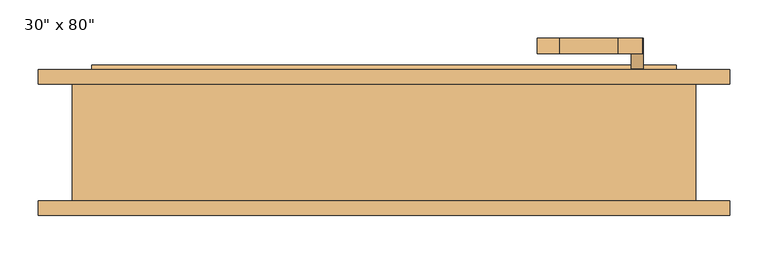
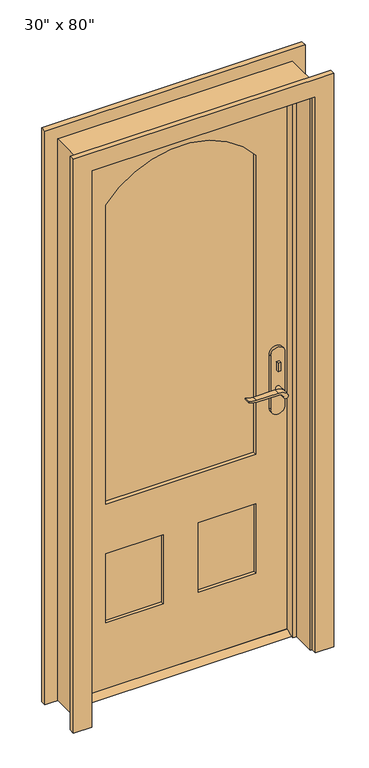
"""IFC4 building model written with IfcOpenShell, lengths in millimetres: door geometry."""

from ifc_helpers import new_model, si_unit, point, frame, frame_2d, origin, place, context, project, spatial, polyline, circle_curve, trimmed, segment, composite_curve, outline, extrude, faceted_brep, source, transform, mapped, element, save


def door_14b9be53(model_context):
    return source(origin(), model_context, "Body", "SolidModel", [
        extrude(outline(polyline([(38.1, 12.7), (73.025, 12.7), (98.425, 0.0), (12.7, 0.0), (38.1, 12.7)])), frame((-381.0, 0.0, 0.0), z_axis=(1.0, 0.0, 0.0), x_axis=(0.0, 1.0, 0.0)), (0.0, 0.0, 1.0), 762.0),
        extrude(outline(polyline([(335.2, 18.1), (325.2, 18.1), (325.2, 28.1), (335.2, 28.1), (335.2, 18.1)])), frame((0.0, 0.0, 981.9), z_axis=(0.0, 0.0, 1.0), x_axis=(1.0, 0.0, 0.0)), (0.0, 0.0, 1.0), 30.0),
        extrude(outline(composite_curve([segment(trimmed(circle_curve(frame_2d((996.9, 330.2)), 8.0), [point((996.9, 322.2))], [point((996.9, 338.2))], False, "CARTESIAN"), True, "CONTINUOUS"), segment(trimmed(circle_curve(frame_2d((996.9, 330.2)), 8.0), [point((996.9, 338.2))], [point((996.9, 322.2))], False, "CARTESIAN"), True, "CONTINUOUS")], self_intersect=False)), frame((0.0, 83.025, 0.0), z_axis=(0.0, 1.0, 0.0), x_axis=(0.0, 0.0, 1.0)), (0.0, 0.0, 1.0), 10.0),
        extrude(outline(composite_curve([segment(trimmed(circle_curve(frame_2d((897.1555521, 306.5324871)), 37.2832219), [point((919.0523287, 336.7081363))], [point((934.4, 304.8325667))], False, "CARTESIAN"), True, "CONTINUOUS"), segment(polyline([(934.4, 304.8325667), (934.4, 228.5564091)]), True, "CONTINUOUS"), segment(trimmed(circle_curve(frame_2d((1017.6850638, 228.6227909)), 83.2850902), [point((934.4, 228.5564091))], [point((939.4, 200.2))], True, "CARTESIAN"), True, "CONTINUOUS"), segment(polyline([(939.4, 200.2), (936.6135558, 200.2)]), True, "CONTINUOUS"), segment(trimmed(circle_curve(frame_2d((986.6709207, 232.1396612)), 59.3791355), [point((936.6135558, 200.2))], [point((927.4, 228.5564091))], False, "CARTESIAN"), True, "CONTINUOUS"), segment(polyline([(927.4, 228.5564091), (927.4, 304.8138099)]), True, "CONTINUOUS"), segment(trimmed(circle_curve(frame_2d((909.2738613, 304.8138099)), 18.1261387), [point((927.4, 304.8138099))], [point((914.4, 322.2))], True, "CARTESIAN"), True, "CONTINUOUS"), segment(trimmed(circle_curve(frame_2d((914.4, 330.2)), 8.0), [point((914.4, 322.2))], [point((919.0523287, 336.7081363))], False, "CARTESIAN"), True, "CONTINUOUS")], self_intersect=False)), frame((0.0, -21.9, 0.0), z_axis=(0.0, 1.0, 0.0), x_axis=(0.0, 0.0, 1.0)), (0.0, 0.0, 1.0), 20.0),
        extrude(outline(composite_curve([segment(trimmed(circle_curve(frame_2d((914.4, 330.2)), 8.0), [point((914.3999903, 322.2))], [point((919.0523287, 336.7081363))], False, "CARTESIAN"), True, "CONTINUOUS"), segment(trimmed(circle_curve(frame_2d((897.1555521, 306.5324871)), 37.2832219), [point((919.0523287, 336.7081363))], [point((934.4, 304.8325667))], False, "CARTESIAN"), True, "CONTINUOUS"), segment(polyline([(934.4, 304.8325667), (934.4, 228.5564091)]), True, "CONTINUOUS"), segment(trimmed(circle_curve(frame_2d((1017.6850638, 228.6227909)), 83.2850902), [point((934.4, 228.5564091))], [point((939.4, 200.2))], True, "CARTESIAN"), True, "CONTINUOUS"), segment(polyline([(939.4, 200.2), (936.6135558, 200.2)]), True, "CONTINUOUS"), segment(trimmed(circle_curve(frame_2d((986.6709207, 232.1396612)), 59.3791355), [point((936.6135558, 200.2))], [point((927.4, 228.5564091))], False, "CARTESIAN"), True, "CONTINUOUS"), segment(polyline([(927.4, 228.5564091), (927.4, 304.8138122)]), True, "CONTINUOUS"), segment(trimmed(circle_curve(frame_2d((909.2738682, 304.8138122)), 18.1261318), [point((927.4, 304.8138122))], [point((914.3999903, 322.2))], True, "CARTESIAN"), True, "CONTINUOUS")], self_intersect=False)), frame((0.0, 113.025, 0.0), z_axis=(0.0, 1.0, 0.0), x_axis=(0.0, 0.0, 1.0)), (0.0, 0.0, 1.0), 20.0),
        extrude(outline(composite_curve([segment(trimmed(circle_curve(frame_2d((914.4, 330.2)), 8.0), [point((914.4, 322.2))], [point((914.4, 338.2))], False, "CARTESIAN"), True, "CONTINUOUS"), segment(trimmed(circle_curve(frame_2d((914.4, 330.2)), 8.0), [point((914.4, 338.2))], [point((914.4, 322.2))], False, "CARTESIAN"), True, "CONTINUOUS")], self_intersect=False)), frame((0.0, -1.9, 0.0), z_axis=(0.0, 1.0, 0.0), x_axis=(0.0, 0.0, 1.0)), (0.0, 0.0, 1.0), 30.0),
        extrude(outline(composite_curve([segment(trimmed(circle_curve(frame_2d((914.4, 330.2)), 8.0), [point((914.4, 322.2))], [point((914.4, 338.2))], False, "CARTESIAN"), True, "CONTINUOUS"), segment(trimmed(circle_curve(frame_2d((914.4, 330.2)), 8.0), [point((914.4, 338.2))], [point((914.4, 322.2))], False, "CARTESIAN"), True, "CONTINUOUS")], self_intersect=False)), frame((0.0, 83.025, 0.0), z_axis=(0.0, 1.0, 0.0), x_axis=(0.0, 0.0, 1.0)), (0.0, 0.0, 1.0), 30.0),
        extrude(outline(composite_curve([segment(polyline([(844.4, 355.2), (1039.4, 355.2)]), True, "CONTINUOUS"), segment(trimmed(circle_curve(frame_2d((1039.4, 330.2)), 25.0), [point((1039.4, 355.2))], [point((1039.4, 305.2))], False, "CARTESIAN"), True, "CONTINUOUS"), segment(polyline([(1039.4, 305.2), (844.4, 305.2)]), True, "CONTINUOUS"), segment(trimmed(circle_curve(frame_2d((844.4, 330.2)), 25.0), [point((844.4, 305.2))], [point((844.4, 355.2))], False, "CARTESIAN"), True, "CONTINUOUS")], self_intersect=False)), frame((0.0, 28.1, 0.0), z_axis=(0.0, 1.0, 0.0), x_axis=(0.0, 0.0, 1.0)), (0.0, 0.0, 1.0), 10.0),
        extrude(outline(composite_curve([segment(polyline([(844.4, 355.2), (1039.4, 355.2)]), True, "CONTINUOUS"), segment(trimmed(circle_curve(frame_2d((1039.4, 330.2)), 25.0), [point((1039.4, 355.2))], [point((1039.4, 305.2))], False, "CARTESIAN"), True, "CONTINUOUS"), segment(polyline([(1039.4, 305.2), (844.4, 305.2)]), True, "CONTINUOUS"), segment(trimmed(circle_curve(frame_2d((844.4, 330.2)), 25.0), [point((844.4, 305.2))], [point((844.4, 355.2))], False, "CARTESIAN"), True, "CONTINUOUS")], self_intersect=False)), frame((0.0, 73.025, 0.0), z_axis=(0.0, 1.0, 0.0), x_axis=(0.0, 0.0, 1.0)), (0.0, 0.0, 1.0), 10.0),
        extrude(outline(polyline([(2032.0, -381.0), (12.7, -381.0), (12.7, 381.0), (2032.0, 381.0), (2032.0, -381.0)]), holes=[composite_curve([segment(polyline([(688.975, -260.35), (1784.35, -260.35)]), True, "CONTINUOUS"), segment(trimmed(circle_curve(frame_2d((1580.99125, 0.0)), 330.35875), [point((1784.35, -260.35))], [point((1784.35, 260.35))], True, "CARTESIAN"), True, "CONTINUOUS"), segment(polyline([(1784.35, 260.35), (688.975, 260.35), (688.975, -260.35)]), True, "CONTINUOUS")], self_intersect=False), polyline([(508.0, -60.325), (254.0, -60.325), (254.0, -260.35), (508.0, -260.35), (508.0, -60.325)]), polyline([(508.0, 260.35), (254.0, 260.35), (254.0, 60.325), (508.0, 60.325), (508.0, 260.35)])]), frame((0.0, 38.1, 0.0), z_axis=(0.0, 1.0, 0.0), x_axis=(0.0, 0.0, 1.0)), (0.0, 0.0, 1.0), 34.925),
        faceted_brep([(406.4, 73.025, 0.0), (406.4, -79.375, 0.0), (381.0, -79.375, 0.0), (381.0, 3.175, 0.0), (368.3, 3.175, 0.0), (368.3, 38.1, 0.0), (381.0, 38.1, 0.0), (381.0, 73.025, 0.0), (406.4, 73.025, 2057.4), (406.4, -79.375, 2057.4), (-406.4, -79.375, 2057.4), (-406.4, -79.375, 0.0), (-381.0, -79.375, 0.0), (-381.0, -79.375, 2032.0), (381.0, -79.375, 2032.0), (381.0, 3.175, 2032.0), (-381.0, 3.175, 2032.0), (-381.0, 3.175, 0.0), (-368.3, 3.175, 0.0), (-368.3, 3.175, 2019.3), (368.3, 3.175, 2019.3), (368.3, 38.1, 2019.3), (-368.3, 38.1, 2019.3), (-368.3, 38.1, 0.0), (-381.0, 38.1, 0.0), (-381.0, 38.1, 2032.0), (381.0, 38.1, 2032.0), (381.0, 73.025, 2032.0), (-381.0, 73.025, 2032.0), (-381.0, 73.025, 0.0), (-406.4, 73.025, 0.0), (-406.4, 73.025, 2057.4)], [[[0, 1, 2, 3, 4, 5, 6, 7]], [[1, 0, 8, 9]], [[2, 1, 9, 10, 11, 12, 13, 14]], [[3, 2, 14, 15]], [[4, 3, 15, 16, 17, 18, 19, 20]], [[5, 4, 20, 21]], [[6, 5, 21, 22, 23, 24, 25, 26]], [[7, 6, 26, 27]], [[0, 7, 27, 28, 29, 30, 31, 8]], [[9, 8, 31, 10]], [[15, 14, 13, 16]], [[21, 20, 19, 22]], [[27, 26, 25, 28]], [[30, 29, 24, 23, 18, 17, 12, 11]], [[10, 31, 30, 11]], [[16, 13, 12, 17]], [[22, 19, 18, 23]], [[28, 25, 24, 29]]]),
        extrude(outline(polyline([(-60.325, 49.7416667), (-260.35, 49.7416667), (-260.35, 61.3833333), (-60.325, 61.3833333), (-60.325, 49.7416667)])), frame((0.0, 0.0, 254.0), z_axis=(0.0, 0.0, 1.0), x_axis=(1.0, 0.0, 0.0)), (0.0, 0.0, 1.0), 254.0),
        extrude(outline(polyline([(260.35, 49.7416667), (60.325, 49.7416667), (60.325, 61.3833333), (260.35, 61.3833333), (260.35, 49.7416667)])), frame((0.0, 0.0, 254.0), z_axis=(0.0, 0.0, 1.0), x_axis=(1.0, 0.0, 0.0)), (0.0, 0.0, 1.0), 254.0),
        extrude(outline(composite_curve([segment(polyline([(688.975, -260.35), (688.975, 260.35), (1784.35, 260.35)]), True, "CONTINUOUS"), segment(trimmed(circle_curve(frame_2d((1580.99125, 0.0)), 330.35875), [point((1784.35, 260.35))], [point((1784.35, -260.35))], False, "CARTESIAN"), True, "CONTINUOUS"), segment(polyline([(1784.35, -260.35), (688.975, -260.35)]), True, "CONTINUOUS")], self_intersect=False)), frame((0.0, 52.07, 0.0), z_axis=(0.0, 1.0, 0.0), x_axis=(0.0, 0.0, 1.0)), (0.0, 0.0, 1.0), 6.985),
        extrude(outline(polyline([(0.0, -450.85), (0.0, -387.35), (2038.35, -387.35), (2038.35, 387.35), (0.0, 387.35), (0.0, 450.85), (2101.85, 450.85), (2101.85, -450.85), (0.0, -450.85)])), frame((0.0, -98.425, 0.0), z_axis=(0.0, 1.0, 0.0), x_axis=(0.0, 0.0, 1.0)), (0.0, 0.0, 1.0), 19.05),
        extrude(outline(polyline([(0.0, -450.85), (0.0, -387.35), (2038.35, -387.35), (2038.35, 387.35), (0.0, 387.35), (0.0, 450.85), (2101.85, 450.85), (2101.85, -450.85), (0.0, -450.85)])), frame((0.0, 73.025, 0.0), z_axis=(0.0, 1.0, 0.0), x_axis=(0.0, 0.0, 1.0)), (0.0, 0.0, 1.0), 19.05),
    ])


if __name__ == "__main__":
    model = new_model("IFC4")
    model_context = context("Model", 3, world=origin())
    ifc_project = project(units=[si_unit("LENGTHUNIT", "METRE", prefix="MILLI")], contexts=[model_context])
    site = spatial("IfcSite", under=ifc_project)
    building = spatial("IfcBuilding", under=site)
    placement = place(None, origin())
    door_shape = door_14b9be53(model_context)
    element("IfcDoor", 1, ObjectType="30\" x 80\"", at=placement, inside=building, context=model_context, shape_type="MappedRepresentation", body=[
        mapped(door_shape, transform((0.0, 0.0, 0.0), x_axis=(1.0, 0.0, 0.0), y_axis=(0.0, 1.0, 0.0), z_axis=(0.0, 0.0, 1.0))),
    ])
    save(model, "model.ifc")

# Revit data of these elements
# Type "30\" x 80\""
#   Type Mark = "9"
#   Assembly Code = "B2030100"
#   Analytic Construction = "French door, wood frame with single glass"
#   Threshold Offset [instance default] = 0' - 0 1/2"
#   Thickness = 0' - 1 3/8"
#   Thermal Resistance (R) = 1.0696 (h·ft²·°F)/BTU
#   Swing Angle [instance default] = 90.00°
#   Stiles = 0' - 4 3/4"
#   Rough Width = 2' - 8"
#   Rough Height = 6' - 9"
#   Radius = 1' - 1.00625"
#   Lock Rail = 0' - 7 1/8"
#   Height = 6' - 8"
#   Width = 2' - 6"
#   Heat Transfer Coefficient (U) = 0.9350 BTU/(h·ft²·°F)
#   Door Offset [instance default] = 0' - 0"
#   Bottom Rail = 0' - 9 1/2"
#   Threshold [instance default] = yes
#   Function = 1
#   Exterior Trim [instance default] = yes
#   Trim Material = Cherry
#   Threshold Material = Cherry
#   Panel Material = Cherry
#   Glazing = Glass
#   Frame Material = Cherry
#   Door Handle Material = Aluminum
#   Visual Light Transmittance = 0
#   Solar Heat Gain Coefficient = 0
#   Wall Closure = (empty or 0)
#   Construction Type = (empty or 0)
# Element 1 (IfcDoor, "30\" x 80\"")
#   Materials on its faces: "Cherry", "Aluminum", "Glass"
# Materials
#   "Cherry": class "Wood", colour RGB 226 177 128, transparency 0, Description = "Prunus Serotina", Cost = 0
#   "Glass": class "Glass", colour RGB 0 128 192, transparency 0.75, Description = "Soda Lime Glass", Cost = 0
#   "Aluminum": class "Metal", colour RGB 247 247 247, transparency 0, Description = "Aluminum 6061", Cost = 0
